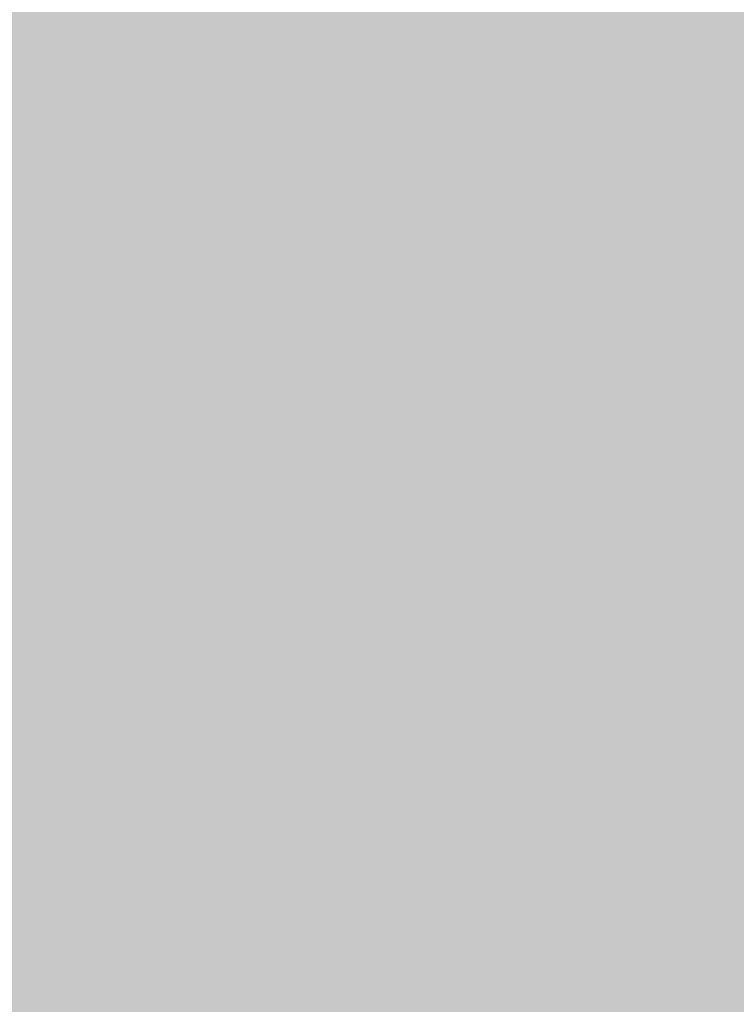
# Model space of a CAD drawing. Units: millimetres. Extents: x -22994 to 29398, y -19990 to 20176.
# Tile 103 of 135: x 231.767 to 237.218, y 79.586 to 87.071. Entities that reach past the tile are written whole.
import ezdxf
from ezdxf import colors
from ezdxf.entities.mleader import LeaderData, LeaderLine
from ezdxf.math import Vec2, Vec3

# ---------------------------------------------------------------- set-up
doc = ezdxf.new("R2010")
doc.units = ezdxf.units.MM
doc.header["$MEASUREMENT"] = 0
doc.layers.add('M-ANNO-TEXT', color=7, linetype='Continuous', lineweight=25)
doc.layers.add('M-DIMS', color=2, linetype='Continuous', lineweight=18)
doc.styles.get("Standard").update_dxf_attribs({"font": 'arial.ttf'})
doc.dimstyles.get("Standard").update_dxf_attribs({"dimtxt": 0.18, "dimasz": 10000, "dimexe": 0.18, "dimexo": 0.0625, "dimgap": 0.09, "dimtad": 0, "dimtih": 1, "dimtoh": 1, "dimdec": 0, "dimzin": 0, "dimdsep": 46, "dimtxsty": 'Standard', "dimcen": 0.09, "dimadec": 0, "dimazin": 0, "dimtfac": 1, "dimtdec": 0, "dimtofl": 0, "dimtmove": 0, "dimatfit": 3, "dimfxl": 1, "dimtolj": 1, "dimtzin": 0, "dimlwd": 30, "dimarcsym": 0})

# ---------------------------------------------------------------- blocks, each defined once
blk = doc.blocks.new('*D2')
at = {"layer": 'Defpoints', "color": 0, "transparency": 16777216}
for p in [(6.6773, 10.2713), (290.852, 10.2713), (290.852, -5.0787)]:
    blk.add_point(p, dxfattribs=at)
at = {"layer": 'M-DIMS', "color": 0, "lineweight": -2, "transparency": 16777216}
for p, q in [((6.6773, 10.2088), (6.6773, -5.2587)), ((290.852, 10.2088), (290.852, -5.2587))]:
    blk.add_line(p, q, dxfattribs=at)
at = {"layer": 'M-DIMS', "color": 0, "lineweight": 30, "transparency": 16777216}
for p, q in [((-9993.3227, -5.0787), (-19993.3227, -5.0787)), ((10290.852, -5.0787), (20290.852, -5.0787))]:
    blk.add_line(p, q, dxfattribs=at)
at = {"layer": 'M-DIMS', "color": 0, "transparency": 16777216}
for points in [[(-9993.3227, 1661.5879), (-9993.3227, -1671.7454), (6.6773, -5.0787)], [(10290.852, 1661.5879), (10290.852, -1671.7454), (290.852, -5.0787)]]:
    blk.add_solid(points, dxfattribs=at)
at = {"layer": 'M-DIMS', "color": 0, "transparency": 16777216, "insert": (148.7647, -5.0787), "char_height": 0.18, "attachment_point": 5}
blk.add_mtext('\\A1;284.2', dxfattribs=at)
blk = doc.blocks.new('*D3')
at = {"layer": 'Defpoints', "color": 0, "transparency": 16777216}
for p in [(110.2647, 204.1654), (110.2647, 176.3662), (95.8327, 127.967)]:
    blk.add_point(p, dxfattribs=at)
at = {"layer": 'M-DIMS', "color": 0, "lineweight": -2, "transparency": 16777216}
for p, q in [((95.8327, 128.0295), (95.8327, 204.3454)), ((110.2647, 176.4287), (110.2647, 204.3454))]:
    blk.add_line(p, q, dxfattribs=at)
at = {"layer": 'M-DIMS', "color": 0, "lineweight": 30, "transparency": 16777216}
for p, q in [((-9904.1673, 204.1654), (-19904.1673, 204.1654)), ((10110.2647, 204.1654), (20110.2647, 204.1654))]:
    blk.add_line(p, q, dxfattribs=at)
at = {"layer": 'M-DIMS', "color": 0, "transparency": 16777216}
for points in [[(-9904.1673, 1870.8321), (-9904.1673, -1462.5013), (95.8327, 204.1654)], [(10110.2647, 1870.8321), (10110.2647, -1462.5013), (110.2647, 204.1654)]]:
    blk.add_solid(points, dxfattribs=at)
at = {"layer": 'M-DIMS', "color": 0, "transparency": 16777216, "insert": (103.0487, 204.1654), "char_height": 0.18, "attachment_point": 5}
blk.add_mtext('\\A1;14.432', dxfattribs=at)
blk = doc.blocks.new('*D4')
at = {"layer": 'Defpoints', "color": 0, "transparency": 16777216}
for p in [(116.2647, 204.1654), (110.2647, 176.3662), (116.2647, 176.3662)]:
    blk.add_point(p, dxfattribs=at)
at = {"layer": 'M-DIMS', "color": 0, "lineweight": -2, "transparency": 16777216}
for p, q in [((110.2647, 176.4287), (110.2647, 204.3454)), ((116.2647, 176.4287), (116.2647, 204.3454))]:
    blk.add_line(p, q, dxfattribs=at)
at = {"layer": 'M-DIMS', "color": 0, "lineweight": 30, "transparency": 16777216}
for p, q in [((-9889.7353, 204.1654), (-19889.7353, 204.1654)), ((10116.2647, 204.1654), (20116.2647, 204.1654))]:
    blk.add_line(p, q, dxfattribs=at)
at = {"layer": 'M-DIMS', "color": 0, "transparency": 16777216}
for points in [[(-9889.7353, 1870.8321), (-9889.7353, -1462.5013), (110.2647, 204.1654)], [(10116.2647, 1870.8321), (10116.2647, -1462.5013), (116.2647, 204.1654)]]:
    blk.add_solid(points, dxfattribs=at)
at = {"layer": 'M-DIMS', "color": 0, "transparency": 16777216, "insert": (113.2647, 204.1654), "char_height": 0.18, "attachment_point": 5}
blk.add_mtext('\\A1;6', dxfattribs=at)
blk = doc.blocks.new('*D5')
at = {"layer": 'Defpoints', "color": 0, "transparency": 16777216}
for p in [(181.2647, 204.1654), (116.2647, 176.3662), (181.2647, 176.3662)]:
    blk.add_point(p, dxfattribs=at)
at = {"layer": 'M-DIMS', "color": 0, "lineweight": -2, "transparency": 16777216}
for p, q in [((116.2647, 176.4287), (116.2647, 204.3454)), ((181.2647, 176.4287), (181.2647, 204.3454))]:
    blk.add_line(p, q, dxfattribs=at)
at = {"layer": 'M-DIMS', "color": 0, "lineweight": 30, "transparency": 16777216}
for p, q in [((-9883.7353, 204.1654), (-19883.7353, 204.1654)), ((10181.2647, 204.1654), (20181.2647, 204.1654))]:
    blk.add_line(p, q, dxfattribs=at)
at = {"layer": 'M-DIMS', "color": 0, "transparency": 16777216}
for points in [[(-9883.7353, 1870.8321), (-9883.7353, -1462.5013), (116.2647, 204.1654)], [(10181.2647, 1870.8321), (10181.2647, -1462.5013), (181.2647, 204.1654)]]:
    blk.add_solid(points, dxfattribs=at)
at = {"layer": 'M-DIMS', "color": 0, "transparency": 16777216, "insert": (148.7647, 204.1654), "char_height": 0.18, "attachment_point": 5}
blk.add_mtext('\\A1;65', dxfattribs=at)
blk = doc.blocks.new('*D6')
at = {"layer": 'Defpoints', "color": 0, "transparency": 16777216}
for p in [(187.2647, 204.1654), (181.2647, 176.3662), (187.2647, 176.3662)]:
    blk.add_point(p, dxfattribs=at)
at = {"layer": 'M-DIMS', "color": 0, "lineweight": -2, "transparency": 16777216}
for p, q in [((181.2647, 176.4287), (181.2647, 204.3454)), ((187.2647, 176.4287), (187.2647, 204.3454))]:
    blk.add_line(p, q, dxfattribs=at)
at = {"layer": 'M-DIMS', "color": 0, "lineweight": 30, "transparency": 16777216}
for p, q in [((-9818.7353, 204.1654), (-19818.7353, 204.1654)), ((10187.2647, 204.1654), (20187.2647, 204.1654))]:
    blk.add_line(p, q, dxfattribs=at)
at = {"layer": 'M-DIMS', "color": 0, "transparency": 16777216}
for points in [[(-9818.7353, 1870.8321), (-9818.7353, -1462.5013), (181.2647, 204.1654)], [(10187.2647, 1870.8321), (10187.2647, -1462.5013), (187.2647, 204.1654)]]:
    blk.add_solid(points, dxfattribs=at)
at = {"layer": 'M-DIMS', "color": 0, "transparency": 16777216, "insert": (184.2647, 204.1654), "char_height": 0.18, "attachment_point": 5}
blk.add_mtext('\\A1;6', dxfattribs=at)
blk = doc.blocks.new('*D7')
at = {"layer": 'Defpoints', "color": 0, "transparency": 16777216}
for p in [(201.6967, 204.1654), (187.2647, 176.3662), (201.6967, 127.967)]:
    blk.add_point(p, dxfattribs=at)
at = {"layer": 'M-DIMS', "color": 0, "lineweight": -2, "transparency": 16777216}
for p, q in [((187.2647, 176.4287), (187.2647, 204.3454)), ((201.6967, 128.0295), (201.6967, 204.3454))]:
    blk.add_line(p, q, dxfattribs=at)
at = {"layer": 'M-DIMS', "color": 0, "lineweight": 30, "transparency": 16777216}
for p, q in [((-9812.7353, 204.1654), (-19812.7353, 204.1654)), ((10201.6967, 204.1654), (20201.6967, 204.1654))]:
    blk.add_line(p, q, dxfattribs=at)
at = {"layer": 'M-DIMS', "color": 0, "transparency": 16777216}
for points in [[(-9812.7353, 1870.8321), (-9812.7353, -1462.5013), (187.2647, 204.1654)], [(10201.6967, 1870.8321), (10201.6967, -1462.5013), (201.6967, 204.1654)]]:
    blk.add_solid(points, dxfattribs=at)
at = {"layer": 'M-DIMS', "color": 0, "transparency": 16777216, "insert": (194.4807, 204.1654), "char_height": 0.18, "attachment_point": 5}
blk.add_mtext('\\A1;14.432', dxfattribs=at)
blk = doc.blocks.new('*D8')
at = {"layer": 'Defpoints', "color": 0, "transparency": 16777216}
for p in [(227.6485, 204.1654), (227.6485, 146.7296), (201.6967, 127.967)]:
    blk.add_point(p, dxfattribs=at)
at = {"layer": 'M-DIMS', "color": 0, "lineweight": -2, "transparency": 16777216}
for p, q in [((201.6967, 128.0295), (201.6967, 204.3454)), ((227.6485, 146.7921), (227.6485, 204.3454))]:
    blk.add_line(p, q, dxfattribs=at)
at = {"layer": 'M-DIMS', "color": 0, "lineweight": 30, "transparency": 16777216}
for p, q in [((-9798.3033, 204.1654), (-19798.3033, 204.1654)), ((10227.6485, 204.1654), (20227.6485, 204.1654))]:
    blk.add_line(p, q, dxfattribs=at)
at = {"layer": 'M-DIMS', "color": 0, "transparency": 16777216}
for points in [[(-9798.3033, 1870.8321), (-9798.3033, -1462.5013), (201.6967, 204.1654)], [(10227.6485, 1870.8321), (10227.6485, -1462.5013), (227.6485, 204.1654)]]:
    blk.add_solid(points, dxfattribs=at)
at = {"layer": 'M-DIMS', "color": 0, "transparency": 16777216, "insert": (214.6726, 204.1654), "char_height": 0.18, "attachment_point": 5}
blk.add_mtext('\\A1;25.95', dxfattribs=at)
blk = doc.blocks.new('*D9')
at = {"layer": 'Defpoints', "color": 0, "transparency": 16777216}
for p in [(187.2647, 176.3662), (306.202, 176.3662), (290.852, 10.2713)]:
    blk.add_point(p, dxfattribs=at)
at = {"layer": 'M-DIMS', "color": 0, "lineweight": 30, "transparency": 16777216}
for p, q in [((306.202, 10176.3662), (306.202, 20176.3662)), ((306.202, -9989.7287), (306.202, -19989.7287))]:
    blk.add_line(p, q, dxfattribs=at)
at = {"layer": 'M-DIMS', "color": 0, "lineweight": -2, "transparency": 16777216}
for p, q in [((187.3272, 176.3662), (306.382, 176.3662)), ((290.9145, 10.2713), (306.382, 10.2713))]:
    blk.add_line(p, q, dxfattribs=at)
at = {"layer": 'M-DIMS', "color": 0, "transparency": 16777216}
for points in [[(-1360.4646, 10176.3662), (1972.8687, 10176.3662), (306.202, 176.3662)], [(-1360.4646, -9989.7287), (1972.8687, -9989.7287), (306.202, 10.2713)]]:
    blk.add_solid(points, dxfattribs=at)
at = {"layer": 'M-DIMS', "color": 0, "transparency": 16777216, "insert": (306.202, 93.3187), "char_height": 0.18, "attachment_point": 5}
blk.add_mtext('\\A1;166.1', dxfattribs=at)
blk = doc.blocks.new('*D10')
at = {"layer": 'Defpoints', "color": 0, "transparency": 16777216}
for p in [(125.6498, 136.0713), (133.3459, 136.0713), (133.3459, -5.0787)]:
    blk.add_point(p, dxfattribs=at)
at = {"layer": 'M-DIMS', "color": 0, "lineweight": -2, "transparency": 16777216}
for p, q in [((125.6498, 136.0088), (125.6498, -5.2587)), ((133.3459, 136.0088), (133.3459, -5.2587))]:
    blk.add_line(p, q, dxfattribs=at)
at = {"layer": 'M-DIMS', "color": 0, "lineweight": 30, "transparency": 16777216}
for p, q in [((-9874.3502, -5.0787), (-19874.3502, -5.0787)), ((10133.3459, -5.0787), (20133.3459, -5.0787))]:
    blk.add_line(p, q, dxfattribs=at)
at = {"layer": 'M-DIMS', "color": 0, "transparency": 16777216}
for points in [[(-9874.3502, 1661.5879), (-9874.3502, -1671.7454), (125.6498, -5.0787)], [(10133.3459, 1661.5879), (10133.3459, -1671.7454), (133.3459, -5.0787)]]:
    blk.add_solid(points, dxfattribs=at)
at = {"layer": 'M-DIMS', "color": 0, "transparency": 16777216, "insert": (129.4978, -5.0787), "char_height": 0.18, "attachment_point": 5}
blk.add_mtext('\\A1;7.696', dxfattribs=at)
blk = doc.blocks.new('*D11')
at = {"layer": 'Defpoints', "color": 0, "transparency": 16777216}
for p in [(133.3459, 136.0713), (135.6498, 136.0713), (135.6498, -5.0787)]:
    blk.add_point(p, dxfattribs=at)
at = {"layer": 'M-DIMS', "color": 0, "lineweight": -2, "transparency": 16777216}
for p, q in [((133.3459, 136.0088), (133.3459, -5.2587)), ((135.6498, 136.0088), (135.6498, -5.2587))]:
    blk.add_line(p, q, dxfattribs=at)
at = {"layer": 'M-DIMS', "color": 0, "lineweight": 30, "transparency": 16777216}
for p, q in [((-9866.6541, -5.0787), (-19866.6541, -5.0787)), ((10135.6498, -5.0787), (20135.6498, -5.0787))]:
    blk.add_line(p, q, dxfattribs=at)
at = {"layer": 'M-DIMS', "color": 0, "transparency": 16777216}
for points in [[(-9866.6541, 1661.5879), (-9866.6541, -1671.7454), (133.3459, -5.0787)], [(10135.6498, 1661.5879), (10135.6498, -1671.7454), (135.6498, -5.0787)]]:
    blk.add_solid(points, dxfattribs=at)
at = {"layer": 'M-DIMS', "color": 0, "transparency": 16777216, "insert": (134.4978, -5.0787), "char_height": 0.18, "attachment_point": 5}
blk.add_mtext('\\A1;2.304', dxfattribs=at)
blk = doc.blocks.new('*D12')
at = {"layer": 'Defpoints', "color": 0, "transparency": 16777216}
for p in [(135.6498, 136.0713), (145.6498, 136.0713), (145.6498, -5.0787)]:
    blk.add_point(p, dxfattribs=at)
at = {"layer": 'M-DIMS', "color": 0, "lineweight": -2, "transparency": 16777216}
for p, q in [((135.6498, 136.0088), (135.6498, -5.2587)), ((145.6498, 136.0088), (145.6498, -5.2587))]:
    blk.add_line(p, q, dxfattribs=at)
at = {"layer": 'M-DIMS', "color": 0, "lineweight": 30, "transparency": 16777216}
for p, q in [((-9864.3502, -5.0787), (-19864.3502, -5.0787)), ((10145.6498, -5.0787), (20145.6498, -5.0787))]:
    blk.add_line(p, q, dxfattribs=at)
at = {"layer": 'M-DIMS', "color": 0, "transparency": 16777216}
for points in [[(-9864.3502, 1661.5879), (-9864.3502, -1671.7454), (135.6498, -5.0787)], [(10145.6498, 1661.5879), (10145.6498, -1671.7454), (145.6498, -5.0787)]]:
    blk.add_solid(points, dxfattribs=at)
at = {"layer": 'M-DIMS', "color": 0, "transparency": 16777216, "insert": (140.6498, -5.0787), "char_height": 0.18, "attachment_point": 5}
blk.add_mtext('\\A1;10', dxfattribs=at)
blk = doc.blocks.new('*D13')
at = {"layer": 'Defpoints', "color": 0, "transparency": 16777216}
for p in [(145.6498, 136.0713), (155.6498, 136.0713), (155.6498, -5.0787)]:
    blk.add_point(p, dxfattribs=at)
at = {"layer": 'M-DIMS', "color": 0, "lineweight": -2, "transparency": 16777216}
for p, q in [((145.6498, 136.0088), (145.6498, -5.2587)), ((155.6498, 136.0088), (155.6498, -5.2587))]:
    blk.add_line(p, q, dxfattribs=at)
at = {"layer": 'M-DIMS', "color": 0, "lineweight": 30, "transparency": 16777216}
for p, q in [((-9854.3502, -5.0787), (-19854.3502, -5.0787)), ((10155.6498, -5.0787), (20155.6498, -5.0787))]:
    blk.add_line(p, q, dxfattribs=at)
at = {"layer": 'M-DIMS', "color": 0, "transparency": 16777216}
for points in [[(-9854.3502, 1661.5879), (-9854.3502, -1671.7454), (145.6498, -5.0787)], [(10155.6498, 1661.5879), (10155.6498, -1671.7454), (155.6498, -5.0787)]]:
    blk.add_solid(points, dxfattribs=at)
at = {"layer": 'M-DIMS', "color": 0, "transparency": 16777216, "insert": (150.6498, -5.0787), "char_height": 0.18, "attachment_point": 5}
blk.add_mtext('\\A1;10', dxfattribs=at)
blk = doc.blocks.new('*D14')
at = {"layer": 'Defpoints', "color": 0, "transparency": 16777216}
for p in [(155.6498, 136.0713), (165.6498, 136.0713), (165.6498, -5.0787)]:
    blk.add_point(p, dxfattribs=at)
at = {"layer": 'M-DIMS', "color": 0, "lineweight": -2, "transparency": 16777216}
for p, q in [((155.6498, 136.0088), (155.6498, -5.2587)), ((165.6498, 136.0088), (165.6498, -5.2587))]:
    blk.add_line(p, q, dxfattribs=at)
at = {"layer": 'M-DIMS', "color": 0, "lineweight": 30, "transparency": 16777216}
for p, q in [((-9844.3502, -5.0787), (-19844.3502, -5.0787)), ((10165.6498, -5.0787), (20165.6498, -5.0787))]:
    blk.add_line(p, q, dxfattribs=at)
at = {"layer": 'M-DIMS', "color": 0, "transparency": 16777216}
for points in [[(-9844.3502, 1661.5879), (-9844.3502, -1671.7454), (155.6498, -5.0787)], [(10165.6498, 1661.5879), (10165.6498, -1671.7454), (165.6498, -5.0787)]]:
    blk.add_solid(points, dxfattribs=at)
at = {"layer": 'M-DIMS', "color": 0, "transparency": 16777216, "insert": (160.6498, -5.0787), "char_height": 0.18, "attachment_point": 5}
blk.add_mtext('\\A1;10', dxfattribs=at)
blk = doc.blocks.new('*D15')
at = {"layer": 'Defpoints', "color": 0, "transparency": 16777216}
for p in [(173.3459, 154.788), (173.3459, 136.0713), (306.202, 136.0713)]:
    blk.add_point(p, dxfattribs=at)
at = {"layer": 'M-DIMS', "color": 0, "lineweight": 30, "transparency": 16777216}
for p, q in [((306.202, 10154.788), (306.202, 20154.788)), ((306.202, -9863.9287), (306.202, -19863.9287))]:
    blk.add_line(p, q, dxfattribs=at)
at = {"layer": 'M-DIMS', "color": 0, "lineweight": -2, "transparency": 16777216}
for p, q in [((173.4084, 154.788), (306.382, 154.788)), ((173.4084, 136.0713), (306.382, 136.0713))]:
    blk.add_line(p, q, dxfattribs=at)
at = {"layer": 'M-DIMS', "color": 0, "transparency": 16777216}
for points in [[(-1360.4646, 10154.788), (1972.8687, 10154.788), (306.202, 154.788)], [(-1360.4646, -9863.9287), (1972.8687, -9863.9287), (306.202, 136.0713)]]:
    blk.add_solid(points, dxfattribs=at)
at = {"layer": 'M-DIMS', "color": 0, "transparency": 16777216, "insert": (306.202, 145.4297), "char_height": 0.18, "attachment_point": 5}
blk.add_mtext('\\A1;18.717', dxfattribs=at)
blk = doc.blocks.new('*D16')
at = {"layer": 'Defpoints', "color": 0, "transparency": 16777216}
for p in [(120.1702, 204.1654), (110.4658, 48.0349), (120.1702, 48.0349)]:
    blk.add_point(p, dxfattribs=at)
at = {"layer": 'M-DIMS', "color": 0, "lineweight": -2, "transparency": 16777216}
for p, q in [((110.4658, 48.0974), (110.4658, 204.3454)), ((120.1702, 48.0974), (120.1702, 204.3454))]:
    blk.add_line(p, q, dxfattribs=at)
at = {"layer": 'M-DIMS', "color": 0, "lineweight": 30, "transparency": 16777216}
for p, q in [((-9889.5342, 204.1654), (-19889.5342, 204.1654)), ((10120.1702, 204.1654), (20120.1702, 204.1654))]:
    blk.add_line(p, q, dxfattribs=at)
at = {"layer": 'M-DIMS', "color": 0, "transparency": 16777216}
for points in [[(-9889.5342, 1870.8321), (-9889.5342, -1462.5013), (110.4658, 204.1654)], [(10120.1702, 1870.8321), (10120.1702, -1462.5013), (120.1702, 204.1654)]]:
    blk.add_solid(points, dxfattribs=at)
at = {"layer": 'M-DIMS', "color": 0, "transparency": 16777216, "insert": (115.318, 204.1654), "char_height": 0.18, "attachment_point": 5}
blk.add_mtext('\\A1;9.704', dxfattribs=at)
blk = doc.blocks.new('*D17')
at = {"layer": 'Defpoints', "color": 0, "transparency": 16777216}
for p in [(126.1702, 204.1654), (120.1702, 48.0349), (126.1702, 48.0349)]:
    blk.add_point(p, dxfattribs=at)
at = {"layer": 'M-DIMS', "color": 0, "lineweight": -2, "transparency": 16777216}
for p, q in [((120.1702, 48.0974), (120.1702, 204.3454)), ((126.1702, 48.0974), (126.1702, 204.3454))]:
    blk.add_line(p, q, dxfattribs=at)
at = {"layer": 'M-DIMS', "color": 0, "lineweight": 30, "transparency": 16777216}
for p, q in [((-9879.8298, 204.1654), (-19879.8298, 204.1654)), ((10126.1702, 204.1654), (20126.1702, 204.1654))]:
    blk.add_line(p, q, dxfattribs=at)
at = {"layer": 'M-DIMS', "color": 0, "transparency": 16777216}
for points in [[(-9879.8298, 1870.8321), (-9879.8298, -1462.5013), (120.1702, 204.1654)], [(10126.1702, 1870.8321), (10126.1702, -1462.5013), (126.1702, 204.1654)]]:
    blk.add_solid(points, dxfattribs=at)
at = {"layer": 'M-DIMS', "color": 0, "transparency": 16777216, "insert": (123.1702, 204.1654), "char_height": 0.18, "attachment_point": 5}
blk.add_mtext('\\A1;6', dxfattribs=at)
blk = doc.blocks.new('*D18')
at = {"layer": 'Defpoints', "color": 0, "transparency": 16777216}
for p in [(132.1702, 204.1654), (126.1702, 48.0349), (132.1702, 48.0349)]:
    blk.add_point(p, dxfattribs=at)
at = {"layer": 'M-DIMS', "color": 0, "lineweight": -2, "transparency": 16777216}
for p, q in [((126.1702, 48.0974), (126.1702, 204.3454)), ((132.1702, 48.0974), (132.1702, 204.3454))]:
    blk.add_line(p, q, dxfattribs=at)
at = {"layer": 'M-DIMS', "color": 0, "lineweight": 30, "transparency": 16777216}
for p, q in [((-9873.8298, 204.1654), (-19873.8298, 204.1654)), ((10132.1702, 204.1654), (20132.1702, 204.1654))]:
    blk.add_line(p, q, dxfattribs=at)
at = {"layer": 'M-DIMS', "color": 0, "transparency": 16777216}
for points in [[(-9873.8298, 1870.8321), (-9873.8298, -1462.5013), (126.1702, 204.1654)], [(10132.1702, 1870.8321), (10132.1702, -1462.5013), (132.1702, 204.1654)]]:
    blk.add_solid(points, dxfattribs=at)
at = {"layer": 'M-DIMS', "color": 0, "transparency": 16777216, "insert": (129.1702, 204.1654), "char_height": 0.18, "attachment_point": 5}
blk.add_mtext('\\A1;6', dxfattribs=at)
blk = doc.blocks.new('*D19')
at = {"layer": 'Defpoints', "color": 0, "transparency": 16777216}
for p in [(138.1702, 204.1654), (132.1702, 48.0349), (138.1702, 48.0349)]:
    blk.add_point(p, dxfattribs=at)
at = {"layer": 'M-DIMS', "color": 0, "lineweight": -2, "transparency": 16777216}
for p, q in [((132.1702, 48.0974), (132.1702, 204.3454)), ((138.1702, 48.0974), (138.1702, 204.3454))]:
    blk.add_line(p, q, dxfattribs=at)
at = {"layer": 'M-DIMS', "color": 0, "lineweight": 30, "transparency": 16777216}
for p, q in [((-9867.8298, 204.1654), (-19867.8298, 204.1654)), ((10138.1702, 204.1654), (20138.1702, 204.1654))]:
    blk.add_line(p, q, dxfattribs=at)
at = {"layer": 'M-DIMS', "color": 0, "transparency": 16777216}
for points in [[(-9867.8298, 1870.8321), (-9867.8298, -1462.5013), (132.1702, 204.1654)], [(10138.1702, 1870.8321), (10138.1702, -1462.5013), (138.1702, 204.1654)]]:
    blk.add_solid(points, dxfattribs=at)
at = {"layer": 'M-DIMS', "color": 0, "transparency": 16777216, "insert": (135.1702, 204.1654), "char_height": 0.18, "attachment_point": 5}
blk.add_mtext('\\A1;6', dxfattribs=at)
blk = doc.blocks.new('*D20')
at = {"layer": 'Defpoints', "color": 0, "transparency": 16777216}
for p in [(144.1702, 204.1654), (138.1702, 48.0349), (144.1702, 48.0349)]:
    blk.add_point(p, dxfattribs=at)
at = {"layer": 'M-DIMS', "color": 0, "lineweight": -2, "transparency": 16777216}
for p, q in [((138.1702, 48.0974), (138.1702, 204.3454)), ((144.1702, 48.0974), (144.1702, 204.3454))]:
    blk.add_line(p, q, dxfattribs=at)
at = {"layer": 'M-DIMS', "color": 0, "lineweight": 30, "transparency": 16777216}
for p, q in [((-9861.8298, 204.1654), (-19861.8298, 204.1654)), ((10144.1702, 204.1654), (20144.1702, 204.1654))]:
    blk.add_line(p, q, dxfattribs=at)
at = {"layer": 'M-DIMS', "color": 0, "transparency": 16777216}
for points in [[(-9861.8298, 1870.8321), (-9861.8298, -1462.5013), (138.1702, 204.1654)], [(10144.1702, 1870.8321), (10144.1702, -1462.5013), (144.1702, 204.1654)]]:
    blk.add_solid(points, dxfattribs=at)
at = {"layer": 'M-DIMS', "color": 0, "transparency": 16777216, "insert": (141.1702, 204.1654), "char_height": 0.18, "attachment_point": 5}
blk.add_mtext('\\A1;6', dxfattribs=at)
blk = doc.blocks.new('*D21')
at = {"layer": 'Defpoints', "color": 0, "transparency": 16777216}
for p in [(149.1157, 204.1654), (144.1702, 48.0349), (149.1157, 48.0349)]:
    blk.add_point(p, dxfattribs=at)
at = {"layer": 'M-DIMS', "color": 0, "lineweight": -2, "transparency": 16777216}
for p, q in [((144.1702, 48.0974), (144.1702, 204.3454)), ((149.1157, 48.0974), (149.1157, 204.3454))]:
    blk.add_line(p, q, dxfattribs=at)
at = {"layer": 'M-DIMS', "color": 0, "lineweight": 30, "transparency": 16777216}
for p, q in [((-9855.8298, 204.1654), (-19855.8298, 204.1654)), ((10149.1157, 204.1654), (20149.1157, 204.1654))]:
    blk.add_line(p, q, dxfattribs=at)
at = {"layer": 'M-DIMS', "color": 0, "transparency": 16777216}
for points in [[(-9855.8298, 1870.8321), (-9855.8298, -1462.5013), (144.1702, 204.1654)], [(10149.1157, 1870.8321), (10149.1157, -1462.5013), (149.1157, 204.1654)]]:
    blk.add_solid(points, dxfattribs=at)
at = {"layer": 'M-DIMS', "color": 0, "transparency": 16777216, "insert": (146.6429, 204.1654), "char_height": 0.18, "attachment_point": 5}
blk.add_mtext('\\A1;4.945', dxfattribs=at)
blk = doc.blocks.new('*D22')
at = {"layer": 'Defpoints', "color": 0, "transparency": 16777216}
for p in [(149.1157, 30.9895), (155.1157, 30.9895), (155.1157, -5.0787)]:
    blk.add_point(p, dxfattribs=at)
at = {"layer": 'M-DIMS', "color": 0, "lineweight": -2, "transparency": 16777216}
for p, q in [((149.1157, 30.927), (149.1157, -5.2587)), ((155.1157, 30.927), (155.1157, -5.2587))]:
    blk.add_line(p, q, dxfattribs=at)
at = {"layer": 'M-DIMS', "color": 0, "lineweight": 30, "transparency": 16777216}
for p, q in [((-9850.8843, -5.0787), (-19850.8843, -5.0787)), ((10155.1157, -5.0787), (20155.1157, -5.0787))]:
    blk.add_line(p, q, dxfattribs=at)
at = {"layer": 'M-DIMS', "color": 0, "transparency": 16777216}
for points in [[(-9850.8843, 1661.5879), (-9850.8843, -1671.7454), (149.1157, -5.0787)], [(10155.1157, 1661.5879), (10155.1157, -1671.7454), (155.1157, -5.0787)]]:
    blk.add_solid(points, dxfattribs=at)
at = {"layer": 'M-DIMS', "color": 0, "transparency": 16777216, "insert": (152.1157, -5.0787), "char_height": 0.18, "attachment_point": 5}
blk.add_mtext('\\A1;6', dxfattribs=at)
blk = doc.blocks.new('*D23')
at = {"layer": 'Defpoints', "color": 0, "transparency": 16777216}
for p in [(155.1157, 30.9895), (161.1157, 30.9895), (161.1157, -5.0787)]:
    blk.add_point(p, dxfattribs=at)
at = {"layer": 'M-DIMS', "color": 0, "lineweight": -2, "transparency": 16777216}
for p, q in [((155.1157, 30.927), (155.1157, -5.2587)), ((161.1157, 30.927), (161.1157, -5.2587))]:
    blk.add_line(p, q, dxfattribs=at)
at = {"layer": 'M-DIMS', "color": 0, "lineweight": 30, "transparency": 16777216}
for p, q in [((-9844.8843, -5.0787), (-19844.8843, -5.0787)), ((10161.1157, -5.0787), (20161.1157, -5.0787))]:
    blk.add_line(p, q, dxfattribs=at)
at = {"layer": 'M-DIMS', "color": 0, "transparency": 16777216}
for points in [[(-9844.8843, 1661.5879), (-9844.8843, -1671.7454), (155.1157, -5.0787)], [(10161.1157, 1661.5879), (10161.1157, -1671.7454), (161.1157, -5.0787)]]:
    blk.add_solid(points, dxfattribs=at)
at = {"layer": 'M-DIMS', "color": 0, "transparency": 16777216, "insert": (158.1157, -5.0787), "char_height": 0.18, "attachment_point": 5}
blk.add_mtext('\\A1;6', dxfattribs=at)
blk = doc.blocks.new('*D24')
at = {"layer": 'Defpoints', "color": 0, "transparency": 16777216}
for p in [(161.1157, 30.9895), (166.4387, 30.9895), (166.4387, -5.0787)]:
    blk.add_point(p, dxfattribs=at)
at = {"layer": 'M-DIMS', "color": 0, "lineweight": -2, "transparency": 16777216}
for p, q in [((161.1157, 30.927), (161.1157, -5.2587)), ((166.4387, 30.927), (166.4387, -5.2587))]:
    blk.add_line(p, q, dxfattribs=at)
at = {"layer": 'M-DIMS', "color": 0, "lineweight": 30, "transparency": 16777216}
for p, q in [((-9838.8843, -5.0787), (-19838.8843, -5.0787)), ((10166.4387, -5.0787), (20166.4387, -5.0787))]:
    blk.add_line(p, q, dxfattribs=at)
at = {"layer": 'M-DIMS', "color": 0, "transparency": 16777216}
for points in [[(-9838.8843, 1661.5879), (-9838.8843, -1671.7454), (161.1157, -5.0787)], [(10166.4387, 1661.5879), (10166.4387, -1671.7454), (166.4387, -5.0787)]]:
    blk.add_solid(points, dxfattribs=at)
at = {"layer": 'M-DIMS', "color": 0, "transparency": 16777216, "insert": (163.7772, -5.0787), "char_height": 0.18, "attachment_point": 5}
blk.add_mtext('\\A1;5.323', dxfattribs=at)
blk = doc.blocks.new('*D25')
at = {"layer": 'Defpoints', "color": 0, "transparency": 16777216}
for p in [(166.4387, 30.9895), (172.4387, 30.9895), (172.4387, -5.0787)]:
    blk.add_point(p, dxfattribs=at)
at = {"layer": 'M-DIMS', "color": 0, "lineweight": -2, "transparency": 16777216}
for p, q in [((166.4387, 30.927), (166.4387, -5.2587)), ((172.4387, 30.927), (172.4387, -5.2587))]:
    blk.add_line(p, q, dxfattribs=at)
at = {"layer": 'M-DIMS', "color": 0, "lineweight": 30, "transparency": 16777216}
for p, q in [((-9833.5613, -5.0787), (-19833.5613, -5.0787)), ((10172.4387, -5.0787), (20172.4387, -5.0787))]:
    blk.add_line(p, q, dxfattribs=at)
at = {"layer": 'M-DIMS', "color": 0, "transparency": 16777216}
for points in [[(-9833.5613, 1661.5879), (-9833.5613, -1671.7454), (166.4387, -5.0787)], [(10172.4387, 1661.5879), (10172.4387, -1671.7454), (172.4387, -5.0787)]]:
    blk.add_solid(points, dxfattribs=at)
at = {"layer": 'M-DIMS', "color": 0, "transparency": 16777216, "insert": (169.4387, -5.0787), "char_height": 0.18, "attachment_point": 5}
blk.add_mtext('\\A1;6', dxfattribs=at)
blk = doc.blocks.new('*D26')
at = {"layer": 'Defpoints', "color": 0, "transparency": 16777216}
for p in [(172.4387, 30.9895), (178.4387, 30.9895), (178.4387, -5.0787)]:
    blk.add_point(p, dxfattribs=at)
at = {"layer": 'M-DIMS', "color": 0, "lineweight": -2, "transparency": 16777216}
for p, q in [((172.4387, 30.927), (172.4387, -5.2587)), ((178.4387, 30.927), (178.4387, -5.2587))]:
    blk.add_line(p, q, dxfattribs=at)
at = {"layer": 'M-DIMS', "color": 0, "lineweight": 30, "transparency": 16777216}
for p, q in [((-9827.5613, -5.0787), (-19827.5613, -5.0787)), ((10178.4387, -5.0787), (20178.4387, -5.0787))]:
    blk.add_line(p, q, dxfattribs=at)
at = {"layer": 'M-DIMS', "color": 0, "transparency": 16777216}
for points in [[(-9827.5613, 1661.5879), (-9827.5613, -1671.7454), (172.4387, -5.0787)], [(10178.4387, 1661.5879), (10178.4387, -1671.7454), (178.4387, -5.0787)]]:
    blk.add_solid(points, dxfattribs=at)
at = {"layer": 'M-DIMS', "color": 0, "transparency": 16777216, "insert": (175.4387, -5.0787), "char_height": 0.18, "attachment_point": 5}
blk.add_mtext('\\A1;6', dxfattribs=at)
blk = doc.blocks.new('*D27')
at = {"layer": 'Defpoints', "color": 0, "transparency": 16777216}
for p in [(178.4387, 30.9895), (188.1175, 30.9895), (188.1175, -5.0787)]:
    blk.add_point(p, dxfattribs=at)
at = {"layer": 'M-DIMS', "color": 0, "lineweight": -2, "transparency": 16777216}
for p, q in [((178.4387, 30.927), (178.4387, -5.2587)), ((188.1175, 30.927), (188.1175, -5.2587))]:
    blk.add_line(p, q, dxfattribs=at)
at = {"layer": 'M-DIMS', "color": 0, "lineweight": 30, "transparency": 16777216}
for p, q in [((-9821.5613, -5.0787), (-19821.5613, -5.0787)), ((10188.1175, -5.0787), (20188.1175, -5.0787))]:
    blk.add_line(p, q, dxfattribs=at)
at = {"layer": 'M-DIMS', "color": 0, "transparency": 16777216}
for points in [[(-9821.5613, 1661.5879), (-9821.5613, -1671.7454), (178.4387, -5.0787)], [(10188.1175, 1661.5879), (10188.1175, -1671.7454), (188.1175, -5.0787)]]:
    blk.add_solid(points, dxfattribs=at)
at = {"layer": 'M-DIMS', "color": 0, "transparency": 16777216, "insert": (183.2781, -5.0787), "char_height": 0.18, "attachment_point": 5}
blk.add_mtext('\\A1;9.679', dxfattribs=at)
blk = doc.blocks.new('*D28')
at = {"layer": 'Defpoints', "color": 0, "transparency": 16777216}
for p in [(188.1175, 48.0349), (306.202, 48.0349), (188.1175, 30.9895)]:
    blk.add_point(p, dxfattribs=at)
at = {"layer": 'M-DIMS', "color": 0, "lineweight": 30, "transparency": 16777216}
for p, q in [((306.202, 10048.0349), (306.202, 20048.0349)), ((306.202, -9969.0105), (306.202, -19969.0105))]:
    blk.add_line(p, q, dxfattribs=at)
at = {"layer": 'M-DIMS', "color": 0, "lineweight": -2, "transparency": 16777216}
for p, q in [((188.18, 48.0349), (306.382, 48.0349)), ((188.18, 30.9895), (306.382, 30.9895))]:
    blk.add_line(p, q, dxfattribs=at)
at = {"layer": 'M-DIMS', "color": 0, "transparency": 16777216}
for points in [[(-1360.4646, 10048.0349), (1972.8687, 10048.0349), (306.202, 48.0349)], [(-1360.4646, -9969.0105), (1972.8687, -9969.0105), (306.202, 30.9895)]]:
    blk.add_solid(points, dxfattribs=at)
at = {"layer": 'M-DIMS', "color": 0, "transparency": 16777216, "insert": (306.202, 39.5122), "char_height": 0.18, "attachment_point": 5}
blk.add_mtext('\\A1;17.045', dxfattribs=at)
blk = doc.blocks.new('*D29')
at = {"layer": 'Defpoints', "color": 0, "transparency": 16777216}
for p in [(36.8006, 80.045), (64.0296, 80.045)]:
    blk.add_point(p, dxfattribs=at)
at = {"layer": 'M-DIMS', "color": 0, "lineweight": -2, "transparency": 16777216}
for p, q in [((50.4151, 79.955), (50.4151, 80.135)), ((50.3251, 80.045), (50.5051, 80.045))]:
    blk.add_line(p, q, dxfattribs=at)
at = {"layer": 'M-DIMS', "color": 0, "lineweight": 30, "transparency": 16777216}
blk.add_line((20064.0296, 80.0303), (10064.0296, 80.0377), dxfattribs=at)
at = {"layer": 'M-DIMS', "color": 0, "transparency": 16777216}
blk.add_solid([(10064.0309, 1746.7043), (10064.0284, -1586.629), (64.0296, 80.045)], dxfattribs=at)
at = {"layer": 'M-DIMS', "color": 0, "transparency": 16777216, "insert": (20064.5213, 80.0303), "char_height": 0.18, "attachment_point": 5}
blk.add_mtext('\\A1;∅27.23', dxfattribs=at)
blk = doc.blocks.new('*D30')
at = {"layer": 'Defpoints', "color": 0, "transparency": 16777216}
for p in [(216.3148, 146.7291), (238.9821, 146.73)]:
    blk.add_point(p, dxfattribs=at)
at = {"layer": 'M-DIMS', "color": 0, "lineweight": 30, "transparency": 16777216}
blk.add_line((20238.9821, 147.4959), (10238.9821, 147.1129), dxfattribs=at)
at = {"layer": 'M-DIMS', "color": 0, "lineweight": -2, "transparency": 16777216}
for p, q in [((227.6485, 146.6396), (227.6485, 146.8196)), ((227.5585, 146.7296), (227.7385, 146.7296))]:
    blk.add_line(p, q, dxfattribs=at)
at = {"layer": 'M-DIMS', "color": 0, "transparency": 16777216}
blk.add_solid([(10238.9183, 1813.7796), (10239.0459, -1519.5537), (238.9821, 146.73)], dxfattribs=at)
at = {"layer": 'M-DIMS', "color": 0, "transparency": 16777216, "insert": (20239.5436, 147.4959), "char_height": 0.18, "attachment_point": 5}
blk.add_mtext('\\A1;∅22.667', dxfattribs=at)
blk = doc.blocks.new('*D31')
at = {"layer": 'Defpoints', "color": 0, "transparency": 16777216}
for p in [(223.1641, 146.7291), (232.1328, 146.73)]:
    blk.add_point(p, dxfattribs=at)
at = {"layer": 'M-DIMS', "color": 0, "lineweight": 30, "transparency": 16777216}
blk.add_line((20232.1327, 148.6656), (10232.1328, 147.6978), dxfattribs=at)
at = {"layer": 'M-DIMS', "color": 0, "lineweight": -2, "transparency": 16777216}
for p, q in [((227.6485, 146.6396), (227.6485, 146.8196)), ((227.5585, 146.7296), (227.7385, 146.7296))]:
    blk.add_line(p, q, dxfattribs=at)
at = {"layer": 'M-DIMS', "color": 0, "transparency": 16777216}
blk.add_solid([(10231.9715, 1814.3645), (10232.2941, -1518.9688), (232.1328, 146.73)], dxfattribs=at)
at = {"layer": 'M-DIMS', "color": 0, "transparency": 16777216, "insert": (20232.6245, 148.6656), "char_height": 0.18, "attachment_point": 5}
blk.add_mtext('\\A1;∅8.969', dxfattribs=at)
blk = doc.blocks.new('*D33')
at = {"layer": 'Defpoints', "color": 0, "transparency": 16777216}
for p in [(229.5613, 154.3773), (232.9972, 153.3509)]:
    blk.add_point(p, dxfattribs=at)
at = {"layer": 'M-DIMS', "color": 0, "lineweight": -2, "transparency": 16777216}
for p, q in [((229.5613, 154.2873), (229.5613, 154.4673)), ((229.4713, 154.3773), (229.6513, 154.3773))]:
    blk.add_line(p, q, dxfattribs=at)
at = {"layer": 'M-DIMS', "color": 0, "lineweight": 30, "transparency": 16777216}
for p, q in [((19396.3388, -5570.8378), (9814.668, -2708.7434)), ((29396.3388, -5570.8378), (19396.3388, -5570.8378))]:
    blk.add_line(p, q, dxfattribs=at)
at = {"layer": 'M-DIMS', "color": 0, "transparency": 16777216}
blk.add_solid([(10291.6837, -1111.7983), (9337.6523, -4305.6886), (232.9972, 153.3509)], dxfattribs=at)
at = {"layer": 'M-DIMS', "color": 0, "transparency": 16777216, "insert": (29397.0125, -5570.8378), "char_height": 0.18, "attachment_point": 5}
blk.add_mtext('\\A1;6X R3.586', dxfattribs=at)
blk = doc.blocks.new('*D36')
at = {"layer": 'Defpoints', "color": 0, "transparency": 16777216}
for p in [(46.39, 31.3035), (46.3875, 26.5934)]:
    blk.add_point(p, dxfattribs=at)
at = {"layer": 'M-DIMS', "color": 0, "lineweight": 30, "transparency": 16777216}
for p, q in [((57.1499, 20031.3006), (51.77, 10031.302)), ((10057.1499, 20031.3006), (57.1499, 20031.3006))]:
    blk.add_line(p, q, dxfattribs=at)
at = {"layer": 'M-DIMS', "color": 0, "lineweight": -2, "transparency": 16777216}
for p, q in [((46.3887, 28.8585), (46.3887, 29.0385)), ((46.2987, 28.9485), (46.4787, 28.9485))]:
    blk.add_line(p, q, dxfattribs=at)
at = {"layer": 'M-DIMS', "color": 0, "transparency": 16777216}
blk.add_solid([(-1614.8965, 10032.1987), (1718.4364, 10030.4054), (46.39, 31.3035)], dxfattribs=at)
at = {"layer": 'M-DIMS', "color": 0, "transparency": 16777216, "insert": (10057.5542, 20031.3006), "char_height": 0.18, "attachment_point": 5}
blk.add_mtext('\\A1;∅4.71', dxfattribs=at)

msp = doc.modelspace()

# ---------------------------------------------------------------- dimensions: what is measured, and where the dimension line sits
at = {"layer": 'M-DIMS'}
for base, p1, p2, override, picture, middle in [((306.202, 176.3662), (290.852, 10.2713), (187.2647, 176.3662), {"dimdec": 1, "dimlfac": 1, "dimrnd": 0, "dimzin": 0, "dimdsep": 46, "dimlunit": 2}, '*D9', (306.202, 93.3187)), ((306.202, 136.0713), (173.3459, 154.788), (173.3459, 136.0713), {"dimdec": 3, "dimlfac": 1, "dimrnd": 0, "dimzin": 0, "dimdsep": 46, "dimlunit": 2}, '*D15', (306.202, 145.4297)), ((306.202, 48.0349), (188.1175, 30.9895), (188.1175, 48.0349), {"dimdec": 3, "dimlfac": 1, "dimrnd": 0, "dimzin": 0, "dimdsep": 46, "dimlunit": 2}, '*D28', (306.202, 39.5122))]:
    dim = msp.add_linear_dim(base=base, p1=p1, p2=p2, angle=90, dimstyle='Standard', override=override, dxfattribs=at)
    dim.commit()
    dim.dimension.update_dxf_attribs({"geometry": picture, "text_midpoint": middle})
for p1, p2, override, picture, middle in [((46.3875, 26.5934), (46.39, 31.3035), {"dimdec": 2, "dimlfac": 1, "dimrnd": 0, "dimzin": 0, "dimdsep": 46, "dimlunit": 2}, '*D36', (10057.5542, 20031.3006)), ((223.1641, 146.7291), (232.1328, 146.73), {"dimdec": 3, "dimlfac": 1, "dimrnd": 0, "dimzin": 0, "dimdsep": 46, "dimlunit": 2}, '*D31', (20232.1327, 148.6656)), ((216.3148, 146.7291), (238.9821, 146.73), {"dimdec": 3, "dimlfac": 1, "dimrnd": 0, "dimzin": 0, "dimdsep": 46, "dimlunit": 2}, '*D30', (20238.9821, 147.4959))]:
    dim = msp.add_diameter_dim_2p(p1=p1, p2=p2, dimstyle='Standard', override=override, dxfattribs=at)
    dim.commit()
    dim.dimension.update_dxf_attribs({"geometry": picture, "text_midpoint": middle, "dimtype": 163})
for base, p1, p2, override, picture, middle in [((110.2647, 204.1654), (95.8327, 127.967), (110.2647, 176.3662), {"dimdec": 3, "dimlfac": 1, "dimrnd": 0, "dimzin": 0, "dimdsep": 46, "dimlunit": 2}, '*D3', (103.0487, 204.1654)), ((116.2647, 204.1654), (110.2647, 176.3662), (116.2647, 176.3662), {"dimdec": 0, "dimlfac": 1, "dimrnd": 0, "dimzin": 0, "dimdsep": 46, "dimlunit": 2}, '*D4', (113.2647, 204.1654)), ((120.1702, 204.1654), (110.4658, 48.0349), (120.1702, 48.0349), {"dimdec": 3, "dimlfac": 1, "dimrnd": 0, "dimzin": 0, "dimdsep": 46, "dimlunit": 2}, '*D16', (115.318, 204.1654)), ((181.2647, 204.1654), (116.2647, 176.3662), (181.2647, 176.3662), {"dimdec": 0, "dimlfac": 1, "dimrnd": 0, "dimzin": 0, "dimdsep": 46, "dimlunit": 2}, '*D5', (148.7647, 204.1654)), ((126.1702, 204.1654), (120.1702, 48.0349), (126.1702, 48.0349), {"dimdec": 0, "dimlfac": 1, "dimrnd": 0, "dimzin": 0, "dimdsep": 46, "dimlunit": 2}, '*D17', (123.1702, 204.1654)), ((132.1702, 204.1654), (126.1702, 48.0349), (132.1702, 48.0349), {"dimdec": 0, "dimlfac": 1, "dimrnd": 0, "dimzin": 0, "dimdsep": 46, "dimlunit": 2}, '*D18', (129.1702, 204.1654)), ((138.1702, 204.1654), (132.1702, 48.0349), (138.1702, 48.0349), {"dimdec": 0, "dimlfac": 1, "dimrnd": 0, "dimzin": 0, "dimdsep": 46, "dimlunit": 2}, '*D19', (135.1702, 204.1654)), ((144.1702, 204.1654), (138.1702, 48.0349), (144.1702, 48.0349), {"dimdec": 0, "dimlfac": 1, "dimrnd": 0, "dimzin": 0, "dimdsep": 46, "dimlunit": 2}, '*D20', (141.1702, 204.1654)), ((149.11567, 204.16539), (144.17023, 48.03494), (149.11567, 48.03494), {"dimdec": 3, "dimlfac": 1, "dimrnd": 0, "dimzin": 0, "dimdsep": 46, "dimlunit": 2}, '*D21', (146.64295, 204.16539)), ((187.2647, 204.1654), (181.2647, 176.3662), (187.2647, 176.3662), {"dimdec": 0, "dimlfac": 1, "dimrnd": 0, "dimzin": 0, "dimdsep": 46, "dimlunit": 2}, '*D6', (184.2647, 204.1654)), ((201.6967, 204.1654), (187.2647, 176.3662), (201.6967, 127.967), {"dimdec": 3, "dimlfac": 1, "dimrnd": 0, "dimzin": 0, "dimdsep": 46, "dimlunit": 2}, '*D7', (194.4807, 204.1654)), ((227.6485, 204.1654), (201.6967, 127.967), (227.6485, 146.7296), {"dimdec": 2, "dimlfac": 1, "dimrnd": 0, "dimzin": 0, "dimdsep": 46, "dimlunit": 2}, '*D8', (214.6726, 204.1654)), ((290.852, -5.0787), (6.6773, 10.2713), (290.852, 10.2713), {"dimdec": 1, "dimlfac": 1, "dimrnd": 0, "dimzin": 0, "dimdsep": 46, "dimlunit": 2}, '*D2', (148.7647, -5.0787)), ((133.3459, -5.0787), (125.6498, 136.0713), (133.3459, 136.0713), {"dimdec": 3, "dimlfac": 1, "dimrnd": 0, "dimzin": 0, "dimdsep": 46, "dimlunit": 2}, '*D10', (129.4978, -5.0787)), ((135.6498, -5.0787), (133.3459, 136.0713), (135.6498, 136.0713), {"dimdec": 3, "dimlfac": 1, "dimrnd": 0, "dimzin": 0, "dimdsep": 46, "dimlunit": 2}, '*D11', (134.4978, -5.0787)), ((145.6498, -5.0787), (135.6498, 136.0713), (145.6498, 136.0713), {"dimdec": 0, "dimlfac": 1, "dimrnd": 0, "dimzin": 0, "dimdsep": 46, "dimlunit": 2}, '*D12', (140.6498, -5.0787)), ((155.6498, -5.0787), (145.6498, 136.0713), (155.6498, 136.0713), {"dimdec": 0, "dimlfac": 1, "dimrnd": 0, "dimzin": 0, "dimdsep": 46, "dimlunit": 2}, '*D13', (150.6498, -5.0787)), ((155.1157, -5.0787), (149.1157, 30.9895), (155.1157, 30.9895), {"dimdec": 0, "dimlfac": 1, "dimrnd": 0, "dimzin": 0, "dimdsep": 46, "dimlunit": 2}, '*D22', (152.1157, -5.0787)), ((161.1157, -5.0787), (155.1157, 30.9895), (161.1157, 30.9895), {"dimdec": 0, "dimlfac": 1, "dimrnd": 0, "dimzin": 0, "dimdsep": 46, "dimlunit": 2}, '*D23', (158.1157, -5.0787)), ((165.6498, -5.0787), (155.6498, 136.0713), (165.6498, 136.0713), {"dimdec": 0, "dimlfac": 1, "dimrnd": 0, "dimzin": 0, "dimdsep": 46, "dimlunit": 2}, '*D14', (160.6498, -5.0787)), ((166.4387, -5.0787), (161.1157, 30.9895), (166.4387, 30.9895), {"dimdec": 3, "dimlfac": 1, "dimrnd": 0, "dimzin": 0, "dimdsep": 46, "dimlunit": 2}, '*D24', (163.7772, -5.0787)), ((172.4387, -5.0787), (166.4387, 30.9895), (172.4387, 30.9895), {"dimdec": 0, "dimlfac": 1, "dimrnd": 0, "dimzin": 0, "dimdsep": 46, "dimlunit": 2}, '*D25', (169.4387, -5.0787)), ((178.4387, -5.0787), (172.4387, 30.9895), (178.4387, 30.9895), {"dimdec": 0, "dimlfac": 1, "dimrnd": 0, "dimzin": 0, "dimdsep": 46, "dimlunit": 2}, '*D26', (175.4387, -5.0787)), ((188.1175, -5.0787), (178.4387, 30.9895), (188.1175, 30.9895), {"dimdec": 3, "dimlfac": 1, "dimrnd": 0, "dimzin": 0, "dimdsep": 46, "dimlunit": 2}, '*D27', (183.2781, -5.0787))]:
    dim = msp.add_linear_dim(base=base, p1=p1, p2=p2, dimstyle='Standard', override=override, dxfattribs=at)
    dim.commit()
    dim.dimension.update_dxf_attribs({"geometry": picture, "text_midpoint": middle})
dim = msp.add_diameter_dim_2p(p1=(36.8006, 80.045), p2=(64.0296, 80.045), dimstyle='Standard', override={"dimdec": 2, "dimlfac": 1, "dimrnd": 0, "dimzin": 0, "dimdsep": 46, "dimlunit": 2}, dxfattribs=at)
dim.commit()
dim.dimension.update_dxf_attribs({"geometry": '*D29', "text_midpoint": (20064.0296, 80.0303)})
dim = msp.add_radius_dim(center=(229.5613, 154.3773), mpoint=(232.9972, 153.3509), text='6X <>', dimstyle='Standard', override={"dimdec": 3, "dimlfac": 1, "dimrnd": 0, "dimzin": 0, "dimdsep": 46, "dimlunit": 2}, dxfattribs=at)
dim.commit()
dim.dimension.update_dxf_attribs({"geometry": '*D33', "text_midpoint": (29397.0125, -5570.8378)})

# ---------------------------------------------------------------- leaders
at = {"layer": 'M-ANNO-TEXT'}
ml = msp.add_multileader_mtext('Standard', dxfattribs=at)
ml.set_content('combustion chamber', color=256)
ml.set_leader_properties()
ml.build(insert=Vec2(0, 0))
ml.multileader.update_dxf_attribs({"dogleg_length": 0.36, "arrow_head_size": 200})
ctx = ml.context
ctx.base_point, ctx.char_height, ctx.arrow_head_size, ctx.landing_gap_size, ctx.plane_origin = Vec3(215.7321, 57.9149), 3, 200, 0.09, Vec3(189.1175, 57.9149)
notes = []
notes.append((ctx, [(0, (1, 1, 0), (215.3721, 57.9149), (1, 0), 0.36, [(0, [(189.1175, 57.9149)], 0, [])])]))
ctx.mtext.insert, ctx.mtext.flow_direction = Vec3(215.8221, 59.4394), 5
for ctx, leaders in notes:
    for number, flags, end, landing, length, lines in leaders:
        leader = LeaderData()
        leader.index, (leader.has_last_leader_line, leader.has_dogleg_vector, leader.attachment_direction) = number, flags
        leader.last_leader_point, leader.dogleg_vector, leader.dogleg_length = Vec3(end), Vec3(landing), length
        for number, points, colour, breaks in lines:
            line = LeaderLine()
            line.index, line.vertices, line.color, line.breaks = number, Vec3.list(points), colors.encode_raw_color(colour), breaks
            leader.lines.append(line)
        ctx.leaders.append(leader)

doc.saveas('drawing.dxf')
